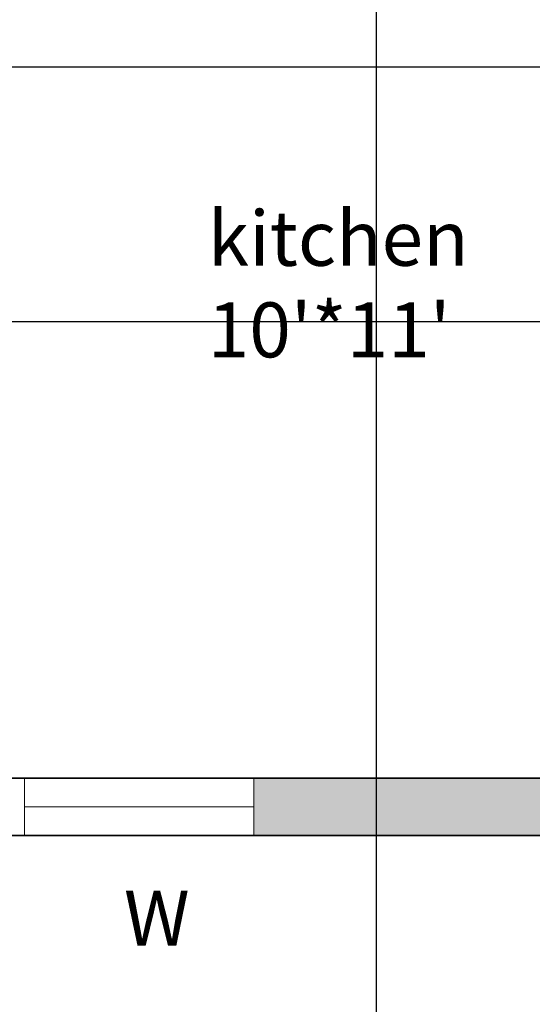
# Model space of a CAD drawing. Units: inches. Extents: x 1568 to 2529, y 2149 to 2897.
# Tile 3 of 16: x 1849 to 1929, y 2304 to 2459. Entities that reach past the tile are written whole.
import ezdxf

# ---------------------------------------------------------------- set-up
doc = ezdxf.new("R2010")
doc.units = ezdxf.units.IN
for name, color, linetype, lineweight in [('A-ANNO-DIMS', 2, 'Continuous', 18), ('A-AREA-IDEN', 210, 'Continuous', 18), ('A-WALL-PATT', 172, 'Continuous', 13), ('text', 210, 'Continuous', 18), ('wall', 7, 'Continuous', 35), ('window', 130, 'Continuous', 18)]:
    doc.layers.add(name, color=color, linetype=linetype, lineweight=lineweight)
doc.styles.get("Standard").update_dxf_attribs({"font": 'arial.ttf'})
doc.dimstyles.get("Standard").update_dxf_attribs({"dimtxt": 0.18, "dimasz": 0.18, "dimexe": 0.18, "dimexo": 0.0625, "dimgap": 0.09, "dimtad": 0, "dimtih": 1, "dimtoh": 1, "dimdec": 4, "dimzin": 0, "dimdsep": 46, "dimtxsty": 'Standard', "dimcen": 0.09, "dimadec": 0, "dimazin": 0, "dimtfac": 1, "dimtdec": 4, "dimtofl": 0, "dimtmove": 0, "dimatfit": 3, "dimfxl": 1, "dimtolj": 1, "dimtzin": 0, "dimarcsym": 0})

# ---------------------------------------------------------------- blocks, each defined once
blk = doc.blocks.new('*D32')
at = {"layer": 'A-ANNO-DIMS', "color": 0, "lineweight": -2, "transparency": 16777216}
for p, q in [((1964.55, 2792.47), (1964.55, 2165.5)), ((1904.55, 2753.4), (1904.55, 2165.5)), ((1904.73, 2165.68), (1934.33, 2165.68)), ((1964.37, 2165.68), (1934.77, 2165.68))]:
    blk.add_line(p, q, dxfattribs=at)
at = {"layer": 'A-ANNO-DIMS', "color": 0, "transparency": 16777216}
for points in [[(1904.73, 2165.71), (1904.73, 2165.65), (1904.55, 2165.68)], [(1964.37, 2165.71), (1964.37, 2165.65), (1964.55, 2165.68)]]:
    blk.add_solid(points, dxfattribs=at)
at = {"layer": 'Defpoints', "color": 0, "transparency": 16777216}
for p in [(1964.55, 2792.53), (1904.55, 2753.46), (1964.55, 2165.68)]:
    blk.add_point(p, dxfattribs=at)
at = {"layer": 'A-ANNO-DIMS', "color": 0, "transparency": 16777216, "insert": (1934.55, 2165.68), "char_height": 0.18, "attachment_point": 5}
blk.add_mtext('\\A1;60', dxfattribs=at)
blk = doc.blocks.new('*D35')
at = {"layer": 'A-ANNO-DIMS', "color": 0, "lineweight": -2, "transparency": 16777216}
for p, q in [((1759.11, 2451.23), (2009.61, 2451.23)), ((2009.43, 2451.05), (2009.43, 2431.41)), ((2009.43, 2411.41), (2009.43, 2431.05)), ((1759.11, 2411.23), (2009.61, 2411.23))]:
    blk.add_line(p, q, dxfattribs=at)
at = {"layer": 'A-ANNO-DIMS', "color": 0, "transparency": 16777216}
for points in [[(2009.4, 2451.05), (2009.46, 2451.05), (2009.43, 2451.23)], [(2009.4, 2411.41), (2009.46, 2411.41), (2009.43, 2411.23)]]:
    blk.add_solid(points, dxfattribs=at)
at = {"layer": 'Defpoints', "color": 0, "transparency": 16777216}
for p in [(1759.05, 2451.23), (2009.43, 2451.23), (1759.05, 2411.23)]:
    blk.add_point(p, dxfattribs=at)
at = {"layer": 'A-ANNO-DIMS', "color": 0, "transparency": 16777216, "insert": (2009.43, 2431.23), "char_height": 0.18, "attachment_point": 5}
blk.add_mtext('\\A1;40', dxfattribs=at)

msp = doc.modelspace()

# ---------------------------------------------------------------- hatches: boundary and pattern name
at = {"layer": 'A-WALL-PATT'}
h = msp.add_hatch(color=256, dxfattribs=at)
h.dxf.hatch_style = 1
h.paths.add_polyline_path([(1738.1593, 2801.532), (1634.4841, 2801.532), (1634.4841, 2792.532), (1738.1593, 2792.532)])
h.paths.add_polyline_path([(1812.4114, 2801.532), (1759.0925, 2801.532), (1759.0925, 2792.532), (1812.4114, 2792.532)])
h.paths.add_polyline_path([(1952.647, 2801.532), (1848.4114, 2801.532), (1848.4114, 2792.532), (1952.647, 2792.532)])
h.paths.add_polyline_path([(1973.5509, 2792.532), (1964.5509, 2792.532), (1964.5509, 2699.1671), (1973.5509, 2699.1671)])
h.paths.add_polyline_path([(1973.5509, 2663.1671), (1964.5509, 2663.1671), (1964.5509, 2630.5978), (1973.5509, 2630.5978)])
h.paths.add_polyline_path([(1973.5509, 2609.6646), (1964.5509, 2609.6646), (1964.5509, 2572.3679), (1973.5509, 2572.3679)])
h.paths.add_polyline_path([(1622.5509, 2753.3576), (1622.3864, 2753.3576), (1613.5509, 2753.3576), (1613.5509, 2705.9172), (1622.5509, 2705.9172)])
h.paths.add_polyline_path([(1622.5509, 2669.9172), (1613.5509, 2669.9172), (1613.5509, 2624.532), (1622.5509, 2624.532)])
h.paths.add_polyline_path([(1759.0509, 2757.9833), (1754.5509, 2757.9833), (1754.5509, 2744.532), (1622.5509, 2744.532), (1622.5509, 2740.032), (1754.5509, 2740.032), (1754.5509, 2730.8156), (1759.0509, 2730.8156), (1759.0509, 2740.032)])
h.paths.add_polyline_path([(1759.0509, 2690.8156), (1754.5509, 2690.8156), (1754.5509, 2624.532), (1759.0509, 2624.532)])
h.paths.add_polyline_path([(1738.1177, 2620.032), (1634.4841, 2620.032), (1634.4841, 2615.532), (1738.1177, 2615.532)])
h.paths.add_polyline_path([(1622.5509, 2615.532), (1613.5509, 2615.532), (1613.5509, 2564.2764), (1622.5509, 2564.2764)])
h.paths.add_polyline_path([(1759.0509, 2411.2271), (1754.5509, 2411.2271), (1754.5509, 2339.532), (1759.0509, 2339.532)])
h.paths.add_polyline_path([(1759.0509, 2464.032), (1734.3925, 2464.032), (1622.5509, 2464.032), (1622.5509, 2459.532), (1736.5509, 2459.532), (1754.5509, 2459.532), (1754.5509, 2451.2271), (1759.0509, 2451.2271)])
h.paths.add_polyline_path([(1844.5509, 2471.532), (1858.1805, 2471.532), (1858.1805, 2476.032), (1844.5509, 2476.032), (1844.5509, 2510.0763), (1840.0509, 2510.0763), (1840.0509, 2476.032), (1840.0509, 2339.532), (1844.5509, 2339.532)])
h.paths.add_polyline_path([(1844.5509, 2596.032), (1964.5509, 2596.032), (1964.5509, 2600.532), (1840.0509, 2600.532), (1840.0509, 2570.0763), (1844.5509, 2570.0763)])
h.paths.add_polyline_path([(1964.5509, 2476.032), (1894.1805, 2476.032), (1894.1805, 2471.532), (1964.5509, 2471.532)])
h.paths.add_polyline_path([(1622.5509, 2528.2764), (1613.5509, 2528.2764), (1613.5509, 2436.512), (1622.5509, 2436.512)])
h.paths.add_polyline_path([(1622.5509, 2400.512), (1613.5509, 2400.512), (1613.5509, 2339.532), (1622.5509, 2339.532)])
h.paths.add_polyline_path([(1738.9144, 2339.532), (1634.4841, 2339.532), (1634.4841, 2330.532), (1738.9144, 2330.532)])
h.paths.add_polyline_path([(1792.463, 2336.532, -0.01876983), (1792.5756, 2339.532), (1783.8928, 2339.532), (1783.8928, 2330.532), (1792.463, 2330.532)])
h.paths.add_polyline_path([(1952.6177, 2339.532), (1885.2912, 2339.532), (1885.2912, 2330.532), (1952.6177, 2330.532)])
h.paths.add_polyline_path([(1973.5509, 2422.371), (1964.5509, 2422.371), (1964.5509, 2395.032), (1964.5509, 2387.286), (1964.5509, 2339.532), (1973.5509, 2339.532)])
h.paths.add_polyline_path([(1973.5509, 2536.3679), (1964.5509, 2536.3679), (1964.5509, 2476.032), (1964.5509, 2458.371), (1973.5509, 2458.371)])

# ---------------------------------------------------------------- linework, layer by layer
at = {"layer": 'wall'}
for p, q in [((1830.713, 2339.532), (1964.5509, 2339.532)), ((1622.5509, 2330.532), (1964.5509, 2330.532))]:
    msp.add_line(p, q, dxfattribs=at)
at = {"layer": 'window'}
for p, q in [((1849.2912, 2339.532), (1849.2912, 2330.532)), ((1885.2912, 2339.532), (1885.2912, 2330.532)), ((1849.2912, 2335.032), (1885.2912, 2335.032))]:
    msp.add_line(p, q, dxfattribs=at)

# ---------------------------------------------------------------- texts
at = {"layer": 'A-AREA-IDEN', "insert": (1878.0636, 2428.6191), "char_height": 8.62815, "attachment_point": 1}
msp.add_mtext_dynamic_manual_height_columns("kitchen\\P10'*11'", width=94.297369, gutter_width=43.1407, heights=[0], dxfattribs=at)
at = {"layer": 'text', "insert": (1864.8951, 2321.8637), "char_height": 8.6281, "attachment_point": 1}
msp.add_mtext_dynamic_manual_height_columns('W', width=94.297369, gutter_width=43.1407, heights=[23.0437], dxfattribs=at)

# ---------------------------------------------------------------- dimensions: what is measured, and where the dimension line sits
at = {"layer": 'A-ANNO-DIMS'}
dim = msp.add_linear_dim(base=(1964.5509, 2165.682), p1=(1904.5509, 2753.4635), p2=(1964.5509, 2792.532), dimstyle='Standard', override={"dimdec": 0, "dimlfac": 1, "dimrnd": 0, "dimzin": 0, "dimdsep": 46, "dimlunit": 2}, dxfattribs=at)
dim.commit()
dim.dimension.update_dxf_attribs({"geometry": '*D32', "text_midpoint": (1934.5509, 2165.682)})
dim = msp.add_linear_dim(base=(2009.4302, 2451.2271), p1=(1759.0509, 2411.2271), p2=(1759.0509, 2451.2271), angle=90, dimstyle='Standard', override={"dimdec": 0, "dimlfac": 1, "dimrnd": 0, "dimzin": 0, "dimdsep": 46, "dimlunit": 2}, dxfattribs=at)
dim.commit()
dim.dimension.update_dxf_attribs({"geometry": '*D35', "text_midpoint": (2009.4302, 2431.2271)})

doc.saveas('drawing.dxf')
